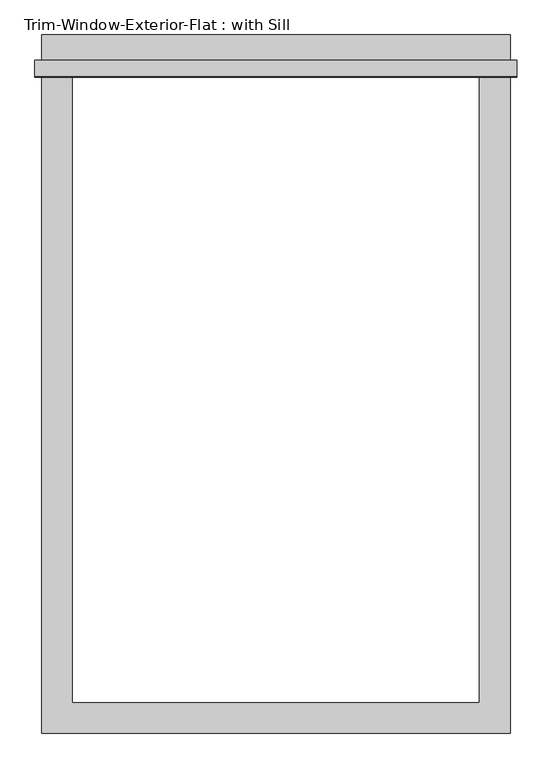
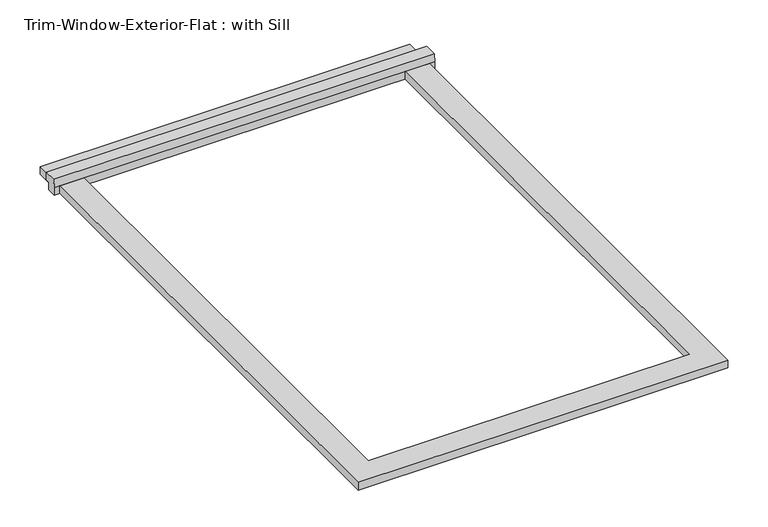
"""IFC4 building model written with IfcOpenShell, lengths in millimetres: proxy geometry, Trim-Window-Exterior-Flat : with Sill."""

from ifc_helpers import new_model, si_unit, frame, origin, origin_with_axes, place, context, project, spatial, polyline, outline, extrude, source, transform, mapped, element, save


def trim_window_exterior_flat_with_sill_e57d6fc0(model_context):
    return source(origin(), model_context, "Body", "SweptSolid", [
        extrude(outline(polyline([(438.15, 1190.5823709), (-438.15, 1190.5823709), (-438.15, 1247.7323709), (438.15, 1247.7323709), (438.15, 1190.5823709)])), origin_with_axes(), (0.0, 0.0, 1.0), 19.05),
        extrude(outline(polyline([(1200.15, 38.1), (1200.15, 19.05), (1190.5823709, 19.05), (1190.5823709, 0.0), (1168.4, 0.0), (1168.4, 19.05), (1170.8580645, 38.1), (1200.15, 38.1)])), frame((-450.85, 0.0, 0.0), z_axis=(1.0, 0.0, 0.0), x_axis=(0.0, 1.0, 0.0)), (0.0, 0.0, 1.0), 901.7),
        extrude(outline(polyline([(-438.15, -57.15), (-438.15, 1168.4), (-381.0, 1168.4), (-381.0, 0.0), (381.0, 0.0), (381.0, 1168.4), (438.15, 1168.4), (438.15, -57.15), (-438.15, -57.15)])), origin_with_axes(), (0.0, 0.0, 1.0), 19.05),
    ])


if __name__ == "__main__":
    model = new_model("IFC4")
    model_context = context("Model", 3, world=origin())
    ifc_project = project(units=[si_unit("LENGTHUNIT", "METRE", prefix="MILLI")], contexts=[model_context])
    site = spatial("IfcSite", under=ifc_project)
    building = spatial("IfcBuilding", under=site)
    placement = place(None, origin())
    trim_window_exterior_flat_with_sill_shape = trim_window_exterior_flat_with_sill_e57d6fc0(model_context)
    element("IfcBuildingElementProxy", 1, Name="Trim-Window-Exterior-Flat : with Sill", ObjectType="Trim-Window-Exterior-Flat : with Sill", at=placement, inside=building, context=model_context, shape_type="MappedRepresentation", body=[
        mapped(trim_window_exterior_flat_with_sill_shape, transform((0.0, 0.0, 0.0), x_axis=(1.0, 0.0, 0.0), y_axis=(0.0, 1.0, 0.0), z_axis=(0.0, 0.0, 1.0))),
    ])
    save(model, "model.ifc")

# Revit data of these elements
# Type "Trim-Window-Exterior-Flat : with Sill"
#   Trim Width = 0' - 2 1/4"
#   Trim Thickness_Picture Frame = 0' - 1 1/4"
#   Trim Thickness_with Sill = 0' - 0 3/4"
#   Sill Thickness = 0' - 1 1/4"
#   Opening Width [instance default] = 2' - 0"
#   Opening Height [instance default] = 3' - 0"
#   Default Elevation = 4' - 0"
#   Sill = yes
#   Picture Frame = no
#   Trim Material [instance default] = none
# Element 1 (IfcBuildingElementProxy, "Trim-Window-Exterior-Flat : with Sill")
#   Opening Width = 2' - 6"
#   Opening Height = 3' - 10"
#   Trim Material = Clad - White
#   Materials on its faces: "Clad - White"
# Materials
#   "Clad - White": class "Wood", colour RGB 242 242 238, transparency 0, Cost = 0
